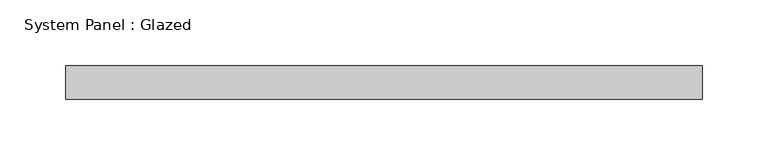
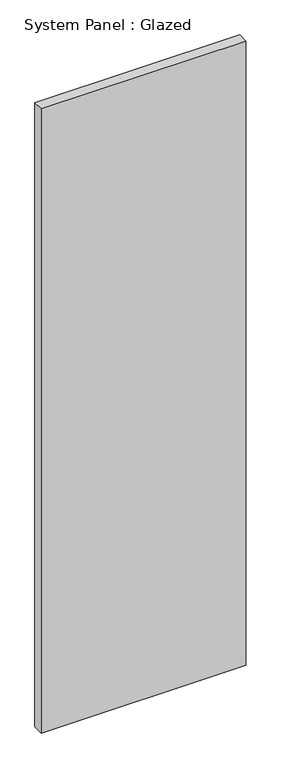
"""IFC4 building model written with IfcOpenShell, lengths in millimetres: plate geometry, System Panel : Glazed."""

from ifc_helpers import new_model, si_unit, origin, origin_with_axes, place, context, project, spatial, polyline, outline, extrude, source, transform, mapped, element, save


def system_panel_glazed_6f1fa804(model_context):
    return source(origin(), model_context, "Body", "SweptSolid", [
        extrude(outline(polyline([(241.3, 19.05), (-241.3, 19.05), (-241.3, 44.45), (241.3, 44.45), (241.3, 19.05)])), origin_with_axes(), (0.0, 0.0, 1.0), 1555.0744644),
    ])


if __name__ == "__main__":
    model = new_model("IFC4")
    model_context = context("Model", 3, world=origin())
    ifc_project = project(units=[si_unit("LENGTHUNIT", "METRE", prefix="MILLI")], contexts=[model_context])
    site = spatial("IfcSite", under=ifc_project)
    building = spatial("IfcBuilding", under=site)
    placement = place(None, origin())
    system_panel_glazed_shape = system_panel_glazed_6f1fa804(model_context)
    element("IfcPlate", 1, ObjectType="System Panel : Glazed", at=placement, inside=building, context=model_context, shape_type="MappedRepresentation", body=[
        mapped(system_panel_glazed_shape, transform((0.0, 0.0, 0.0), x_axis=(1.0, 0.0, 0.0), y_axis=(0.0, 1.0, 0.0), z_axis=(0.0, 0.0, 1.0))),
    ])
    save(model, "model.ifc")

# Revit data of these elements
# Type "System Panel : Glazed"
#   Construction Type Id = "GSP4R"
#   Analytic Construction = "1/8 in Pilkington single glazing"
#   Visual Light Transmittance = 0.9
#   Solar Heat Gain Coefficient = 0.86
#   Heat Transfer Coefficient (U) = 1.18115 BTU/(h·ft²·°F)
#   Define Thermal Properties by = 1
# Element 1 (IfcPlate, "System Panel : Glazed")
#   Materials on its faces: "Glass"
# Materials
#   "Glass": class "Glass", colour RGB 0 128 192, transparency 0.75, Description = "Soda Lime Glass", Cost = 0
